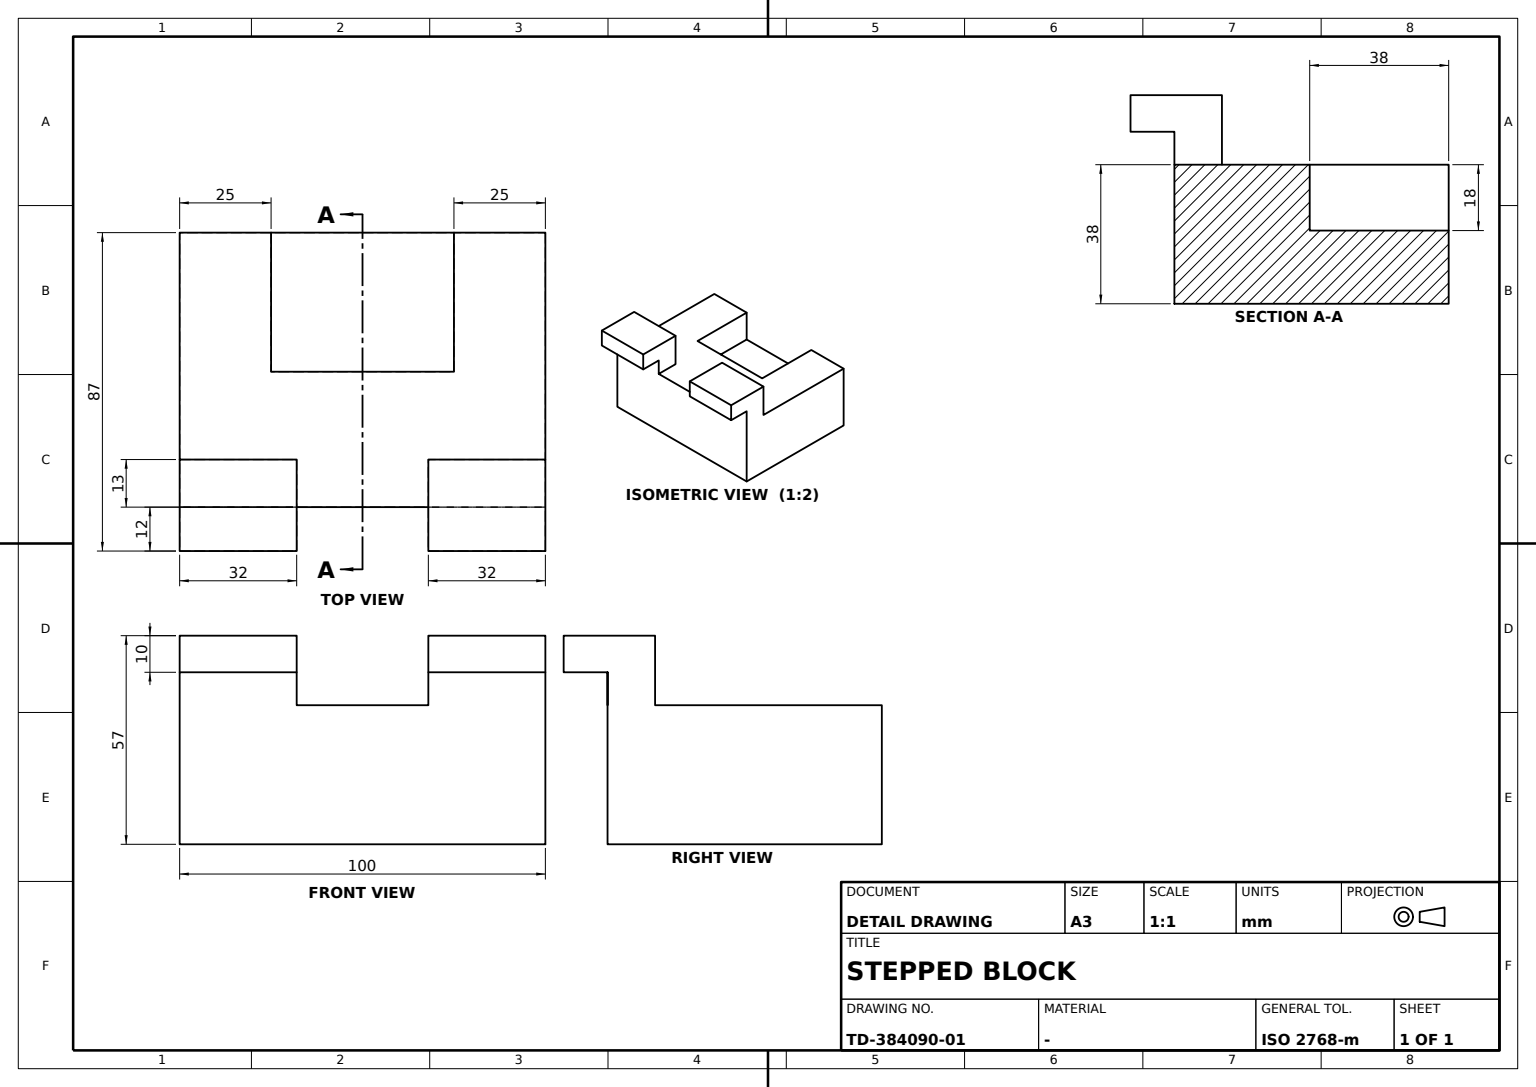
CATIA V5 part; units mm, degrees
sketch "Sketch1" plane through (0, 0, 0) normal (0, 0, 1) x (1, 0, 0)
  line L0 (50, 37.5) -> (-50, 37.5)
  line L1 (-50, 37.5) -> (-50, -37.5)
  line L2 (-50, -37.5) -> (50, -37.5)
  line L3 (50, -37.5) -> (50, 37.5)
  dimension "length L1" = 75
  dimension "length L2" = 100
  constraint horizontal L0 x-axis
  constraint horizontal L2 x-axis
  constraint vertical L1 y-axis
  constraint vertical L3 y-axis
  constraint symmetry L3 L1 y-axis
  constraint symmetry L0 L2 x-axis
extrude "Pad1" add sketch "Sketch1" along normal blind 38
sketch "Sketch2" plane through (0, 0, 38) normal (0, 0, 1) x (1, 0, 0)
  line L0 (50, 37.5) -> (-50, 37.5) construction
  line L1 (25, 37.5) -> (-25, 37.5)
  point P0 (-25, 37.5)
  line L2 (-25, 37.5) -> (-25, -0.5)
  line L3 (-25, -0.5) -> (25, -0.5)
  line L4 (25, -0.5) -> (25, 37.5)
  line L5 (50, -37.5) -> (50, 37.5) construction
  line L6 (-50, 37.5) -> (-50, -37.5) construction
  dimension "distance L4 L5" = 25
  dimension "distance L6 L2" = 25
  dimension "length L2" = 38
  constraint vertical L2 y-axis
  constraint vertical L4 y-axis
  constraint horizontal L3 x-axis
  constraint coincidence P0 L0
extrude "Pocket1" cut sketch "Sketch2" against normal blind 18
sketch "Sketch3" plane through (50, 0, 0) normal (1, 0, 0) x (0, 1, 0)
  line L0 (-24.5, 38) -> (-24.5, 57)
  line L1 (-24.5, 57) -> (-49.5, 57)
  line L2 (-49.5, 57) -> (-49.5, 47)
  line L3 (-49.5, 47) -> (-37.5, 47)
  line L4 (-37.5, 47) -> (-37.5, 38)
  point P0 (-37.5, 38)
  line L5 (-37.5, 38) -> (-24.5, 38)
  point P1 (-37.5, 38)
  point P2 (-37.5, 38)
  dimension "length L0" = 19
  dimension "length L1" = 25
  dimension "length L3" = 12
  constraint vertical L0 y-axis
  constraint vertical L2 y-axis
  constraint vertical L4 y-axis
  constraint horizontal L1 x-axis
  constraint horizontal L3 x-axis
  constraint horizontal L5 x-axis
  constraint coincidence P1 L5
  constraint coincidence P0 P2
extrude "Pad2" add sketch "Sketch3" against normal blind 32
mirror "Mirror1" about plane through (0, 0, 0) normal (1, 0, 0) of "Pad2"
